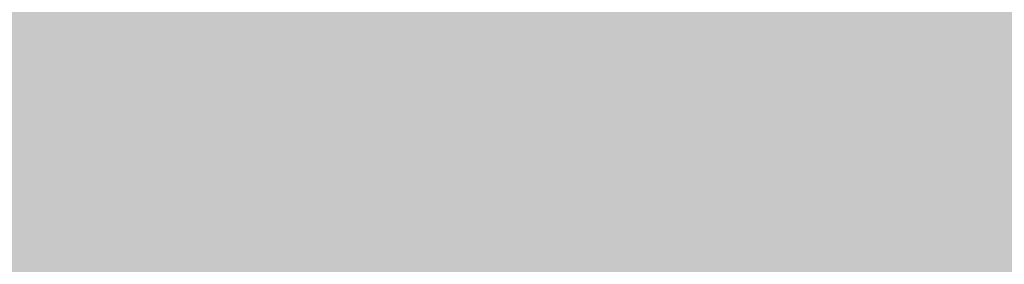
# Model space of a CAD drawing. Units: inches. Extents: x 2083 to 3317, y 1141 to 2115.
# Tile 158 of 256: x 3126.955939 to 3126.958245, y 1263.261932 to 1263.262504. Entities that reach past the tile are written whole.
import ezdxf

# ---------------------------------------------------------------- set-up
doc = ezdxf.new("R2010")
doc.units = ezdxf.units.IN
doc.layers.add('A-ANNO-DIMS', color=2, linetype='Continuous', lineweight=18)
doc.layers.add('A-WALL-PATT', color=251, linetype='Continuous', lineweight=13, true_color=0x636466)
doc.styles.get("Standard").update_dxf_attribs({"font": 'arial.ttf'})
doc.dimstyles.new('ISO-25', dxfattribs={"dimtxt": 12, "dimasz": 12, "dimexe": 1.25, "dimexo": 0.625, "dimtad": 1, "dimlunit": 3, "dimtxsty": 'Standard', "dimcen": 2.5, "dimadec": 0, "dimazin": 0, "dimtfac": 1, "dimtmove": 0, "dimatfit": 3, "dimfxl": 1, "dimarcsym": 0})

# ---------------------------------------------------------------- blocks, each defined once
blk = doc.blocks.new('*D26')
at = {"layer": 'A-ANNO-DIMS', "color": 0, "lineweight": -2, "transparency": 16777216}
for p, q in [((3088.985844, 1274.915092), (3088.985844, 1270.9519631)), ((3111.2400366, 1274.915092), (3111.2400366, 1270.9519631)), ((3076.985844, 1272.2019631), (2840.262447, 1272.2019631)), ((3111.2400366, 1272.2019631), (3088.985844, 1272.2019631)), ((3123.2400366, 1272.2019631), (3135.2400366, 1272.2019631))]:
    blk.add_line(p, q, dxfattribs=at)
at = {"layer": 'A-ANNO-DIMS', "color": 0, "transparency": 16777216}
for points in [[(3076.985844, 1274.2019631), (3076.985844, 1270.2019631), (3088.985844, 1272.2019631)], [(3123.2400366, 1274.2019631), (3123.2400366, 1270.2019631), (3111.2400366, 1272.2019631)]]:
    blk.add_solid(points, dxfattribs=at)
at = {"layer": 'Defpoints', "color": 0, "transparency": 16777216}
for p in [(3088.985844, 1275.540092), (3111.2400366, 1275.540092), (3088.985844, 1272.2019631)]:
    blk.add_point(p, dxfattribs=at)
at = {"layer": 'A-ANNO-DIMS', "color": 0, "transparency": 16777216, "insert": (2952.6241455, 1279.0316016), "char_height": 12, "attachment_point": 5}
blk.add_mtext('NIGHTSTAND 1\'-10 1/2" TYP.', dxfattribs=at)

msp = doc.modelspace()

# ---------------------------------------------------------------- hatches: boundary and pattern name
at = {"layer": 'A-WALL-PATT'}
h = msp.add_hatch(color=256, dxfattribs=at)
h.dxf.hatch_style = 1
h.paths.add_polyline_path([(3126.9597832, 2020.7613601), (2748.9597832, 2020.7613601), (2604.9597832, 2020.7613601), (2226.9597832, 2020.7613601), (2226.9597832, 1702.7613601), (2466.9597832, 1702.7613601), (2466.9597832, 1582.7613601), (2418.9597832, 1582.7613601), (2418.9597832, 1477.7613601), (2226.9597832, 1477.7613601), (2226.9597832, 1263.2613601), (2544.9597832, 1263.2613601), (2544.9597832, 1411.7613601), (2604.9597832, 1411.7613601), (2685.9597832, 1411.7613601), (2685.9597832, 1420.7613601), (2604.9597832, 1420.7613601), (2604.9597832, 1573.7613601), (2604.9597832, 1702.7613601), (2604.9597832, 2011.7613601), (2748.9597832, 2011.7613601), (2748.9597832, 1702.7613601), (2862.9597832, 1702.7613601), (2862.9597832, 1621.7613601), (2871.9597832, 1621.7613601), (2871.9597832, 1702.7613601), (2883.9597832, 1702.7613601), (2883.9597832, 1706.9394595, -0.026459), (2883.9597832, 1711.7613601), (2757.9597832, 1711.7613601), (2757.9597832, 1807.7613601), (2787.9597832, 1807.7613601), (2787.9597832, 1812.2613601), (2757.9597832, 1812.2613601), (2757.9597832, 2011.7613601), (2877.9597832, 2011.7613601), (2877.9597832, 1812.2613601), (2847.9597832, 1812.2613601), (2847.9597832, 1807.7613601), (2889.8357425, 1807.7613601), (2889.8357425, 1812.2613601), (2882.4597832, 1812.2613601), (2882.4597832, 2011.7613601), (3117.9597832, 2011.7613601), (3117.9597832, 1812.2613601), (2937.8357425, 1812.2613601), (2937.8357425, 1807.7613601), (2995.7097832, 1807.7613601), (2995.7097832, 1796.1176655), (3000.2097832, 1796.1176655), (3000.2097832, 1807.7613601), (3117.9597832, 1807.7613601), (3117.9597832, 1711.7613601), (3000.2097832, 1711.7613601), (3000.2097832, 1760.1176655), (2998.5727047, 1760.1176655, -0.020711), (2995.7097832, 1760.1176655), (2995.7097832, 1711.7613601), (2931.9597832, 1711.7613601), (2931.9597832, 1702.7613601), (3126.9597832, 1702.7613601)])
h.paths.add_polyline_path([(2471.4597832, 2011.7613601), (2471.4597832, 1810.0113601), (2462.7169357, 1810.0113601), (2462.7169357, 1805.5113601), (2505.9597832, 1805.5113601), (2505.9597832, 1810.0113601), (2475.9597832, 1810.0113601), (2475.9597832, 2011.7613601), (2595.9597832, 2011.7613601), (2595.9597832, 1810.0113601), (2565.9597832, 1810.0113601), (2565.9597832, 1805.5113601), (2595.9597832, 1805.5113601), (2595.9597832, 1711.7613601), (2235.9597832, 1711.7613601), (2235.9597832, 1805.5113601), (2353.7097832, 1805.5113601), (2353.7097832, 1796.0541624), (2358.2097832, 1796.0541624), (2358.2097832, 1805.5113601), (2414.7169357, 1805.5113601), (2414.7169357, 1810.0113601), (2235.9597832, 1810.0113601), (2235.9597832, 2011.7613601)], flags=16)
h.paths.add_polyline_path([(2270.2047343, 1994.6100082), (2270.2047343, 1970.6100082), (2246.2047343, 1970.6100082), (2246.2047343, 1994.6100082)], flags=0)
edge = h.paths.add_edge_path(flags=0)
edge.add_ellipse((2332.027391, 1899.7981761), major_axis=(-3.0429938, 3.0429938), ratio=0.16825245, start_angle=-161.3321656, end_angle=-156.3071136, ccw=False)
edge.add_ellipse((2333.0820373, 1898.7435297), major_axis=(-1.0546463, 1.0546463), ratio=0.453532097, start_angle=-123.371019, end_angle=-94.1591066)
edge = h.paths.add_edge_path(flags=0)
edge.add_ellipse((2332.027391, 1968.8762897), major_axis=(3.0429938, 3.0429938), ratio=0.16825245, start_angle=18.6678344, end_angle=23.6928864)
edge.add_spline(control_points=[(2332.9255964, 1970.6911045), (2332.2267681, 1970.3360997), (2330.8937087, 1969.6589054), (2328.4130803, 1970.9321376), (2327.2039345, 1967.7487119), (2324.7095965, 1969.9555886), (2322.5328223, 1967.012354), (2320.0128462, 1971.2958124), (2317.6803077, 1968.1578449), (2316.0405263, 1967.1020468), (2315.4269045, 1966.8096022)], knot_values=[0, 0, 0, 0, 2.267059, 4.324559, 6.685584, 8.878641, 11.121502, 14.300359, 17.755284, 19.732645, 19.732645, 19.732645, 19.732645], degree=3, periodic=0)
edge.add_ellipse((2332.027391, 1968.8762897), major_axis=(3.0429938, 3.0429938), ratio=0.16825245, start_angle=18.6678344, end_angle=23.6928864, ccw=False)
edge.add_ellipse((2333.0820373, 1969.930936), major_axis=(1.0546463, 1.0546463), ratio=0.453532097, start_angle=56.628981, end_angle=85.8408934, ccw=False)
edge = h.paths.add_edge_path(flags=0)
edge.add_spline(control_points=[(2296.4282874, 1967.9879081), (2293.6278045, 1965.3363137), (2287.7036238, 1959.727094), (2299.7438601, 1949.9956993), (2294.5325909, 1935.6685275), (2290.5732281, 1920.6035119), (2293.3941244, 1909.9736911), (2296.1854073, 1904.9665431)], knot_values=[0.099185, 0.099185, 0.099185, 0.099185, 0.345301, 0.619822, 0.982653, 1.386093, 1.810555, 1.810555, 1.810555, 1.810555], degree=3, periodic=0)
edge.add_spline(control_points=[(2296.1854073, 1904.9665431), (2297.3835817, 1902.6193002), (2298.0009694, 1901.9493116), (2298.5529698, 1901.4681549)], knot_values=[0.006246, 0.006246, 0.006246, 0.006246, 0.055476, 0.055476, 0.055476, 0.055476], degree=3, periodic=0)
edge.add_spline(control_points=[(2298.5529698, 1901.4681549), (2297.2586121, 1900.9232238), (2295.2252939, 1900.2321257), (2293.0602287, 1900.6142053), (2292.1014227, 1900.788415), (2292.0895776, 1900.790568)], knot_values=[0.312835, 0.312835, 0.312835, 0.312835, 0.40178, 0.474987, 0.475903, 0.475903, 0.475903, 0.475903], degree=3, periodic=0)
edge.add_arc((2292.7936464, 1904.6641088), 3.9370079, 215.4208969, 259.6981795, ccw=False)
edge.add_spline(control_points=[(2289.5853139, 1902.3823039), (2289.4766524, 1902.5350874), (2289.3684805, 1902.6880353), (2289.2608648, 1902.8411699)], knot_values=[0.102872, 0.102872, 0.102872, 0.102872, 0.116896, 0.116896, 0.116896, 0.116896], degree=3, periodic=0)
edge.add_spline(control_points=[(2289.2608648, 1902.8411699), (2288.6866042, 1902.5501922), (2287.6400477, 1902.0199025), (2285.8813368, 1901.8739536), (2283.8529717, 1901.5043521), (2281.7199871, 1899.7105375), (2278.4669913, 1899.492942), (2276.1571361, 1901.8832022), (2272.2589526, 1899.8040711), (2267.7776054, 1901.8431828), (2262.2438819, 1900.1840326), (2257.414927, 1901.7820606), (2254.318374, 1900.7261196), (2253.1782849, 1900.3373431)], knot_values=[0, 0, 0, 0, 1.907977, 3.477176, 5.261074, 7.972851, 11.680248, 13.717921, 16.939592, 22.789562, 27.502503, 33.595215, 37.145618, 37.145618, 37.145618, 37.145618], degree=3, periodic=0)
edge.add_line((2253.1782849, 1900.3373431), (2250.2442397, 1902.8411699))
edge.add_line((2250.2442397, 1902.8411699), (2250.2442397, 1965.8332959))
edge.add_line((2250.2442397, 1965.8332959), (2253.1782849, 1968.3371226))
edge.add_spline(control_points=[(2253.1782849, 1968.3371226), (2254.318374, 1967.9483462), (2257.414927, 1966.8924051), (2262.2438819, 1968.4904332), (2267.7776054, 1966.8312829), (2271.5267301, 1968.5372172), (2273.8759143, 1967.8282895), (2274.2067012, 1967.7276424)], knot_values=[0, 0, 0, 0, 0.09018, 0.244935, 0.364644, 0.513233, 0.537855, 0.537855, 0.537855, 0.537855], degree=3, periodic=0)
edge.add_arc((2274.3528869, 1963.7933495), 3.9370079, 72.0511336, 92.1279492, ccw=False)
edge.add_arc((2281.2969331, 1985.2300027), 18.5962982, 252.05113361, 288.56572166)
edge.add_arc((2292.3167172, 1956.0288805), 12.6460805, 71.02678788, 113.77821843, ccw=False)
edge = h.paths.add_edge_path(flags=0)
edge.add_spline(control_points=[(2274.8994147, 1951.8561946), (2275.066156, 1951.6165924), (2275.2326866, 1951.3765878), (2275.3979871, 1951.1358545)], knot_values=[1.409916, 1.409916, 1.409916, 1.409916, 1.43159, 1.43159, 1.43159, 1.43159], degree=3, periodic=0)
edge.add_spline(control_points=[(2275.3979871, 1951.1358545), (2275.7921055, 1950.5618854), (2276.1792311, 1949.9837745), (2276.5455462, 1949.3971029)], knot_values=[1.358238, 1.358238, 1.358238, 1.358238, 1.409916, 1.409916, 1.409916, 1.409916], degree=3, periodic=0)
edge.add_line((2276.5455462, 1949.3971029), (2277.437289, 1947.8621847))
edge.add_spline(control_points=[(2277.437289, 1947.8621847), (2276.3038341, 1945.6731147), (2274.6396979, 1942.4268817), (2274.631615, 1938.0938998), (2272.7991237, 1930.8515498), (2274.3564261, 1943.8970461), (2275.9476814, 1947.9233558), (2276.5455462, 1949.3971029)], knot_values=[0.005632, 0.005632, 0.005632, 0.005632, 0.186014, 0.266002, 0.357087, 0.59639, 0.739732, 0.739732, 0.739732, 0.739732], degree=3, periodic=0)
edge.add_spline(control_points=[(2276.5455462, 1949.3971029), (2276.1792311, 1949.9837745), (2275.7921055, 1950.5618854), (2275.3979871, 1951.1358545)], knot_values=[1.358238, 1.358238, 1.358238, 1.358238, 1.409916, 1.409916, 1.409916, 1.409916], degree=3, periodic=0)
edge.add_spline(control_points=[(2275.3979871, 1951.1358545), (2274.9425002, 1950.0804523), (2274.2077604, 1948.0252718), (2273.9346018, 1944.8514774), (2272.4685341, 1937.6274891), (2273.4662155, 1945.6964663), (2274.7006154, 1951.0594725), (2274.8994147, 1951.8561946)], knot_values=[0.104364, 0.104364, 0.104364, 0.104364, 0.189636, 0.269624, 0.36071, 0.600013, 0.644622, 0.644622, 0.644622, 0.644622], degree=3, periodic=0)
h.paths.add_polyline_path([(2269.1675139, 1963.1275729, -0.357527), (2268.170633, 1960.9763695, -0.092561), (2268.170633, 1939.4363249, -0.357527), (2269.1675139, 1937.2851215, -0.357527), (2267.0163105, 1938.2820024, -0.164785), (2254.6855813, 1938.2820024, -0.357527), (2252.5343779, 1937.2851215, -0.357527), (2253.5312587, 1939.4363249, -0.092561), (2253.5312587, 1960.9763695, -0.357527), (2252.5343779, 1963.1275729, -0.357527), (2254.6855813, 1962.130692, -0.164785), (2267.0163105, 1962.130692, -0.357527)], flags=0)
h.paths.add_polyline_path([(2248.8740679, 1967.8017998), (2248.8740679, 1957.0277095), (2249.4577833, 1957.0277095), (2249.4577833, 1911.6467562), (2248.8740679, 1911.6467562), (2248.8740679, 1900.8726659), (2246.5118632, 1900.8726659, 0.197327), (2244.1496584, 1902.4568734), (2244.1496584, 1966.2175923, 0.197327), (2246.5118632, 1967.8017998)], flags=0)
h.paths.add_polyline_path([(2269.1675139, 1931.3893442, -0.357527), (2268.170633, 1929.2381408, -0.092561), (2268.170633, 1907.6980962, -0.357527), (2269.1675139, 1905.5468928, -0.357527), (2267.0163105, 1906.5437737, -0.164785), (2254.6855813, 1906.5437737, -0.357527), (2252.5343779, 1905.5468928, -0.357527), (2253.5312587, 1907.6980962, -0.092561), (2253.5312587, 1929.2381408, -0.357527), (2252.5343779, 1931.3893442, -0.357527), (2254.6855813, 1930.3924634, -0.164785), (2267.0163105, 1930.3924634, -0.357527)], flags=0)
edge = h.paths.add_edge_path(flags=0)
edge.add_spline(control_points=[(2276.1968578, 1906.7237016), (2276.1681442, 1909.0289278), (2276.1140492, 1913.371852), (2270.5984171, 1924.9249783), (2273.9051746, 1919.0127787), (2275.9217115, 1916.2620626), (2275.4745699, 1912.4021495), (2277.2578735, 1910.3806206), (2276.6960436, 1908.2250358), (2276.6462176, 1906.8130226), (2276.6178249, 1906.0084068)], knot_values=[0, 0, 0, 0, 8.61026, 16.221274, 18.843057, 23.804898, 27.440828, 29.356102, 31.203478, 33.650687, 33.650687, 33.650687, 33.650687], degree=3, periodic=0)
edge.add_spline(control_points=[(2276.6178249, 1906.0084068), (2276.6233131, 1905.6241436), (2276.4977381, 1904.6286608), (2275.4417789, 1903.8547251), (2274.9373144, 1903.0804497), (2274.8590804, 1902.8411699)], knot_values=[0.156488, 0.156488, 0.156488, 0.156488, 0.184398, 0.231376, 0.250598, 0.250598, 0.250598, 0.250598], degree=3, periodic=0)
edge.add_line((2274.8590804, 1902.8411699), (2276.50598, 1902.8411699))
edge.add_spline(control_points=[(2276.50598, 1902.8411699), (2276.7883084, 1903.0849395), (2277.6650711, 1904.1251958), (2278.2495378, 1904.340738), (2277.6538719, 1908.5273866), (2278.15567, 1906.2278078), (2278.100464, 1905.2859484), (2278.8466748, 1904.0690054), (2277.8567853, 1903.4149482), (2277.8741909, 1902.9910497), (2277.9035616, 1902.8411699)], knot_values=[0.059574, 0.059574, 0.059574, 0.059574, 0.080753, 0.103741, 0.16972, 0.176036, 0.207137, 0.240474, 0.262341, 0.27366, 0.27366, 0.27366, 0.27366], degree=3, periodic=0)
edge.add_line((2277.9035616, 1902.8411699), (2280.0298255, 1902.8411699))
edge.add_spline(control_points=[(2280.0298255, 1902.8411699), (2279.8882214, 1903.088398), (2279.4992571, 1903.9815512), (2280.1522839, 1905.9393491), (2278.103615, 1909.6577572), (2279.7623946, 1907.185285), (2280.3279002, 1904.8748608), (2280.4851086, 1903.4895904), (2281.4632687, 1903.2494323), (2281.7583431, 1902.9364967), (2281.8340361, 1902.8411699)], knot_values=[0.013856, 0.013856, 0.013856, 0.013856, 0.034874, 0.088867, 0.107879, 0.126738, 0.158714, 0.193757, 0.217487, 0.226722, 0.226722, 0.226722, 0.226722], degree=3, periodic=0)
edge.add_spline(control_points=[(2281.8340361, 1902.8411699), (2281.7875348, 1902.8267029), (2281.6470224, 1902.7829881), (2281.3955272, 1902.85949), (2281.088077, 1902.9852418), (2280.7206826, 1903.060902), (2280.3334513, 1903.0257257), (2280.1247668, 1902.898879), (2280.0298255, 1902.8411699)], knot_values=[0, 0, 0, 0, 0.14413, 0.435517, 0.749276, 1.153046, 1.548371, 1.878348, 1.878348, 1.878348, 1.878348], degree=3, periodic=0)
edge.add_line((2280.0298255, 1902.8411699), (2277.9035616, 1902.8411699))
edge.add_spline(control_points=[(2277.9035616, 1902.8411699), (2277.892855, 1902.7958553), (2277.865396, 1902.6796374), (2277.6074793, 1902.6874828), (2277.2740503, 1902.8006999), (2276.8379209, 1902.6197745), (2276.5838074, 1902.7892611), (2276.50598, 1902.8411699)], knot_values=[0, 0, 0, 0, 0.127189, 0.326199, 0.628009, 1.24357, 1.515331, 1.515331, 1.515331, 1.515331], degree=3, periodic=0)
edge.add_line((2276.50598, 1902.8411699), (2274.8590804, 1902.8411699))
edge.add_spline(control_points=[(2274.8590804, 1902.8411699), (2274.8144367, 1902.8985868), (2274.7251297, 1903.013446), (2274.4934765, 1903.1189684), (2274.2442854, 1902.9605386), (2273.9371207, 1903.1849416), (2273.6140395, 1902.9831428), (2273.4083164, 1902.8830449), (2273.322254, 1902.8411699)], knot_values=[0, 0, 0, 0, 0.21843, 0.436957, 0.687977, 0.990379, 1.398396, 1.69185, 1.69185, 1.69185, 1.69185], degree=3, periodic=0)
edge.add_spline(control_points=[(2273.322254, 1902.8411699), (2273.6167403, 1903.445692), (2274.2739977, 1904.5382529), (2276.0272387, 1904.5737017), (2276.2069634, 1906.5836372), (2276.1968578, 1906.7237016)], knot_values=[0.012227, 0.012227, 0.012227, 0.012227, 0.059472, 0.106218, 0.134458, 0.134458, 0.134458, 0.134458], degree=3, periodic=0)
h.paths.add_polyline_path([(2270.7760538, 1897.7898284), (2270.7760538, 1873.7898284), (2246.7760538, 1873.7898284), (2246.7760538, 1897.7898284)], flags=0)
h.paths.add_polyline_path([(2353.7097832, 1760.0050593), (2353.7097832, 1760.0541624), (2358.2097832, 1760.0541624, -0.033729)], flags=0)
h.paths.add_polyline_path([(2321.8191188, 1737.5291862), (2341.9953271, 1737.5291862, -0.414214), (2343.2032727, 1736.3212406), (2343.2032727, 1721.0205964, -0.414214), (2341.9953271, 1719.8126508), (2321.8191188, 1719.8126508, -0.414214), (2320.6111732, 1721.0205964), (2320.6111732, 1736.3212406, -0.414214)], flags=0)
h.paths.add_polyline_path([(2324.2350099, 1736.3212406), (2339.5794359, 1736.3212406, -0.414214), (2341.9953271, 1733.9053494), (2341.9953271, 1725.4497302, -0.414214), (2339.5794359, 1723.033839), (2333.6805885, 1723.033839), (2333.8453172, 1722.0454666, -0.870646), (2335.4253988, 1721.8258934, -0.767327), (2333.922694, 1721.4232449), (2331.2910241, 1721.4232449, -0.767327), (2329.7883193, 1721.8258934, -0.870646), (2331.3684009, 1722.0454666), (2331.5331296, 1723.033839), (2324.2350099, 1723.033839, -0.414214), (2321.8191188, 1725.4497302), (2321.8191188, 1733.9053494, -0.414214)], flags=0)
h.paths.add_polyline_path([(2570.4837892, 1928.6154443), (2589.6837892, 1928.6154443), (2590.1688286, 1928.6154443), (2590.1688286, 1904.9933971), (2570.4837892, 1904.9933971)], flags=0)
h.paths.add_polyline_path([(2574.4473242, 1927.2638215, -1), (2572.8288357, 1927.2638215, -1)], flags=0)
h.paths.add_polyline_path([(2573.0898665, 1926.9408768), (2573.925032, 1927.7760423), (2574.1477428, 1927.5533315), (2573.3125773, 1926.718166)], flags=0)
h.paths.add_polyline_path([(2578.7790648, 1919.7296175, -1), (2571.5916632, 1919.7296175, -1)], flags=0)
h.paths.add_polyline_path([(2578.385364, 1919.7296175, -1), (2571.985364, 1919.7296175, -1)], flags=0)
h.paths.add_polyline_path([(2331.5957638, 1729.4762156, -1), (2333.6179542, 1729.4762156, -1)], flags=0)
h.paths.add_polyline_path([(2578.0342282, 1927.2638215, -1), (2576.4157396, 1927.2638215, -1)], flags=0)
h.paths.add_polyline_path([(2576.6888513, 1927.5310886), (2576.9115621, 1927.7537993), (2577.7467276, 1926.9186339), (2577.5240168, 1926.6959231)], flags=0)
h.paths.add_polyline_path([(2578.1390648, 1909.8595388, -1), (2572.2316632, 1909.8595388, -1)], flags=0)
h.paths.add_polyline_path([(2577.745364, 1909.8595388, -1), (2572.625364, 1909.8595388, -1)], flags=0)
h.paths.add_polyline_path([(2583.7977179, 1927.2638215, -1), (2582.1792294, 1927.2638215, -1)], flags=0)
h.paths.add_polyline_path([(2582.7186487, 1927.7537993), (2583.5538142, 1926.9186339), (2583.3311034, 1926.6959231), (2582.4959379, 1927.5310886)], flags=0)
h.paths.add_polyline_path([(2582.4959379, 1927.5310886), (2582.7186487, 1927.7537993), (2583.5538142, 1926.9186339), (2583.3311034, 1926.6959231)], flags=0)
h.paths.add_polyline_path([(2587.7390648, 1920.5296175, -1), (2581.8316632, 1920.5296175, -1)], flags=0)
h.paths.add_polyline_path([(2587.345364, 1920.5296175, -1), (2582.225364, 1920.5296175, -1)], flags=0)
h.paths.add_polyline_path([(2587.3846219, 1927.2638215, -1), (2585.7661333, 1927.2638215, -1)], flags=0)
h.paths.add_polyline_path([(2586.0819925, 1926.9802469), (2586.917158, 1927.8154124), (2587.1398688, 1927.5927016), (2586.3047033, 1926.7575361)], flags=0)
h.paths.add_polyline_path([(2588.3790648, 1910.6595388, -1), (2581.1916632, 1910.6595388, -1)], flags=0)
h.paths.add_polyline_path([(2587.985364, 1910.6595388, -1), (2581.585364, 1910.6595388, -1)], flags=0)
h.paths.add_polyline_path([(2417.1677288, 1729.4778955), (2437.3439372, 1729.4778955, -0.414214), (2438.5518828, 1728.2699499), (2438.5518828, 1712.9693057, -0.414214), (2437.3439372, 1711.7613601), (2417.1677288, 1711.7613601, -0.414214), (2415.9597832, 1712.9693057), (2415.9597832, 1728.2699499, -0.414214)], flags=0)
h.paths.add_polyline_path([(2419.58362, 1728.2699499), (2434.928046, 1728.2699499, -0.414214), (2437.3439372, 1725.8540587), (2437.3439372, 1717.3984395, -0.414214), (2434.928046, 1714.9825483), (2429.0291985, 1714.9825483), (2429.1939273, 1713.9941758, -0.870646), (2430.7740089, 1713.7746027, -0.767327), (2429.2713041, 1713.3719542), (2426.6396342, 1713.3719542, -0.767327), (2425.1369294, 1713.7746027, -0.870646), (2426.717011, 1713.9941758), (2426.8817397, 1714.9825483), (2419.58362, 1714.9825483, -0.414214), (2417.1677288, 1717.3984395), (2417.1677288, 1725.8540587, -0.414214)], flags=0)
h.paths.add_polyline_path([(2419.58362, 1728.2699499), (2434.928046, 1728.2699499, -0.414214), (2437.3439372, 1725.8540587), (2437.3439372, 1717.3984395, -0.414214), (2434.928046, 1714.9825483), (2429.0291985, 1714.9825483), (2428.3581177, 1719.0090337), (2427.5528206, 1719.0090337), (2426.8817397, 1714.9825483), (2419.58362, 1714.9825483, -0.414214), (2417.1677288, 1717.3984395), (2417.1677288, 1725.8540587, -0.414214)], flags=0)
h.paths.add_polyline_path([(2426.9443739, 1721.4249248, -1), (2428.9665643, 1721.4249248, -1)], flags=0)
h.paths.add_polyline_path([(2475.9597832, 1702.7613601), (2595.9597832, 1702.7613601), (2595.9597832, 1582.7613601), (2475.9597832, 1582.7613601)], flags=16)
h.paths.add_polyline_path([(2427.9597832, 1573.7613601), (2595.9597832, 1573.7613601), (2595.9597832, 1468.7613601), (2595.9597832, 1420.7613601), (2384.4597832, 1420.7613601), (2384.4597832, 1468.7613601), (2427.9597832, 1468.7613601)], flags=16)
h.paths.add_polyline_path([(2379.9597832, 1468.7613601), (2379.9597832, 1420.7613601), (2235.9597832, 1420.7613601), (2235.9597832, 1468.7613601)], flags=16)
h.paths.add_polyline_path([(2317.8159962, 1466.695767), (2337.9922045, 1466.695767, -0.414214), (2339.2001501, 1465.4878214), (2339.2001501, 1450.1871771, -0.414214), (2337.9922045, 1448.9792315), (2317.8159962, 1448.9792315, -0.414214), (2316.6080506, 1450.1871771), (2316.6080506, 1465.4878214, -0.414214)], flags=0)
h.paths.add_polyline_path([(2320.2318874, 1465.4878214), (2335.5763133, 1465.4878214, -0.414214), (2337.9922045, 1463.0719302), (2337.9922045, 1454.616311, -0.414214), (2335.5763133, 1452.2004198), (2329.6774659, 1452.2004198), (2329.8421946, 1451.2120473, -0.870646), (2331.4222762, 1450.9924742, -0.767327), (2329.9195714, 1450.5898257), (2327.2879015, 1450.5898257, -0.767327), (2325.7851967, 1450.9924742, -0.870646), (2327.3652783, 1451.2120473), (2327.530007, 1452.2004198), (2320.2318874, 1452.2004198, -0.414214), (2317.8159962, 1454.616311), (2317.8159962, 1463.0719302, -0.414214)], flags=0)
h.paths.add_polyline_path([(2320.2318874, 1465.4878214), (2335.5763133, 1465.4878214, -0.414214), (2337.9922045, 1463.0719302), (2337.9922045, 1454.616311, -0.414214), (2335.5763133, 1452.2004198), (2329.6774659, 1452.2004198), (2329.006385, 1456.2269051), (2328.2010879, 1456.2269051), (2327.530007, 1452.2004198), (2320.2318874, 1452.2004198, -0.414214), (2317.8159962, 1454.616311), (2317.8159962, 1463.0719302, -0.414214)], flags=0)
h.paths.add_polyline_path([(2327.5926413, 1458.6427963, -1), (2329.6148317, 1458.6427963, -1)], flags=0)
h.paths.add_polyline_path([(2244.4117436, 1433.3404531), (2241.9209449, 1433.3404531, -0.414214), (2240.0178562, 1435.2435418), (2240.0178562, 1440.9528078, -0.414211), (2241.920925, 1442.8558965), (2244.4117436, 1442.8558965, -1.976472)], flags=0)
h.paths.add_polyline_path([(2245.3568884, 1434.3975358, -0.414214), (2245.3568884, 1441.7988138, -2.144098)], flags=0)
h.paths.add_polyline_path([(2535.9597832, 1416.2613601), (2535.9597832, 1272.2613601), (2235.9597832, 1272.2613601), (2235.9597832, 1416.2613601)], flags=16)
h.paths.add_polyline_path([(2260.1195614, 1384.2928413), (2260.1195614, 1362.0386487), (2237.8653688, 1362.0386487), (2237.8653688, 1384.2928413)], flags=0)
edge = h.paths.add_edge_path(flags=0)
edge.add_line((2318.2518466, 1362.0932983), (2318.1457968, 1362.0009726))
edge.add_ellipse((2317.4451158, 1360.4310442), major_axis=(2.8216404, 2.8216404), ratio=0.16825245, start_angle=18.6678344, end_angle=20.9481273, ccw=False)
edge.add_ellipse((2318.4230451, 1361.4089735), major_axis=(0.9779293, 0.9779293), ratio=0.453532097, start_angle=56.628981, end_angle=70.2262012, ccw=False)
edge = h.paths.add_edge_path(flags=0)
edge.add_line((2319.1073699, 1295.5710784), (2319.0150442, 1295.6771282))
edge.add_ellipse((2317.4451158, 1296.3778091), major_axis=(-2.8216404, 2.8216404), ratio=0.16825245, start_angle=-161.3321656, end_angle=-159.0518727, ccw=False)
edge.add_ellipse((2318.4230451, 1295.3998798), major_axis=(-0.9779293, 0.9779293), ratio=0.453532097, start_angle=-123.371019, end_angle=-109.7737988)
edge = h.paths.add_edge_path(flags=0)
edge.add_spline(control_points=[(2284.2103489, 1301.1702189), (2284.5806878, 1300.444719), (2284.8911891, 1299.8920243), (2285.159553, 1299.4610182)], knot_values=[0.039066, 0.039066, 0.039066, 0.039066, 0.055476, 0.055476, 0.055476, 0.055476], degree=3, periodic=0)
edge.add_line((2285.159553, 1299.4610182), (2284.2103489, 1301.1702189))
edge = h.paths.add_edge_path(flags=0)
edge.add_line((2280.4124579, 1297.2980125), (2283.3699905, 1297.0361216))
edge.add_line((2283.3699905, 1297.0361216), (2286.4056902, 1297.9263104))
edge.add_spline(control_points=[(2286.4056902, 1297.9263104), (2285.305487, 1297.4631193), (2284.3447774, 1297.1291508), (2283.3699905, 1297.0361216)], knot_values=[0.394369, 0.394369, 0.394369, 0.394369, 0.475903, 0.475903, 0.475903, 0.475903], degree=3, periodic=0)
edge.add_spline(control_points=[(2283.3699905, 1297.0361216), (2283.2813895, 1297.027666), (2282.316289, 1296.9573356), (2281.3125019, 1297.1344787), (2280.4234414, 1297.2960161), (2280.4124579, 1297.2980125)], knot_values=[0.312835, 0.312835, 0.312835, 0.312835, 0.320246, 0.393453, 0.394369, 0.394369, 0.394369, 0.394369], degree=3, periodic=0)
edge = h.paths.add_edge_path(flags=0)
edge.add_line((2284.4355615, 1359.6072854), (2280.4462909, 1355.328047))
edge.add_line((2280.4462909, 1355.328047), (2279.5799868, 1351.0177544))
edge.add_line((2279.5799868, 1351.0177544), (2282.4129737, 1346.5804327))
edge.add_spline(control_points=[(2282.4129737, 1346.5804327), (2283.1533308, 1345.5892358), (2284.2528957, 1344.0288973), (2284.801037, 1342.3871671), (2284.9351625, 1341.8055443)], knot_values=[1.240098, 1.240098, 1.240098, 1.240098, 1.332892, 1.382712, 1.382712, 1.382712, 1.382712], degree=3, periodic=0)
edge.add_spline(control_points=[(2284.9351625, 1341.8055443), (2285.3191079, 1340.1406002), (2285.2330291, 1338.4092041), (2284.9099384, 1336.6541222)], knot_values=[1.097484, 1.097484, 1.097484, 1.097484, 1.240098, 1.240098, 1.240098, 1.240098], degree=3, periodic=0)
edge.add_spline(control_points=[(2284.9099384, 1336.6541222), (2284.5868478, 1334.8990403), (2284.0267453, 1333.1202725), (2283.4626437, 1331.3605849)], knot_values=[0.95487, 0.95487, 0.95487, 0.95487, 1.097484, 1.097484, 1.097484, 1.097484], degree=3, periodic=0)
edge.add_line((2283.4626437, 1331.3605849), (2281.8903759, 1326.153357))
edge.add_line((2281.8903759, 1326.153357), (2280.7562592, 1321.0560888))
edge.add_line((2280.7562592, 1321.0560888), (2280.2992048, 1316.0019772))
edge.add_line((2280.2992048, 1316.0019772), (2280.7159327, 1310.9500678))
edge.add_line((2280.7159327, 1310.9500678), (2282.0280939, 1305.9721367))
edge.add_line((2282.0280939, 1305.9721367), (2284.2103489, 1301.1702189))
edge.add_spline(control_points=[(2284.2103489, 1301.1702189), (2283.3407305, 1302.7301854), (2282.6119044, 1304.3364933), (2282.0280939, 1305.9721367)], knot_values=[0.099185, 0.099185, 0.099185, 0.099185, 0.241799, 0.241799, 0.241799, 0.241799], degree=3, periodic=0)
edge.add_spline(control_points=[(2282.0280939, 1305.9721367), (2281.4442835, 1307.6077801), (2281.0054886, 1309.2727591), (2280.7159327, 1310.9500678)], knot_values=[0.241799, 0.241799, 0.241799, 0.241799, 0.384413, 0.384413, 0.384413, 0.384413], degree=3, periodic=0)
edge.add_spline(control_points=[(2280.7159327, 1310.9500678), (2280.4332411, 1312.5876134), (2280.2893863, 1314.2769594), (2280.2988938, 1315.9620324), (2280.2992048, 1316.0019772)], knot_values=[0.384413, 0.384413, 0.384413, 0.384413, 0.523647, 0.527028, 0.527028, 0.527028, 0.527028], degree=3, periodic=0)
edge.add_spline(control_points=[(2280.2992048, 1316.0019772), (2280.3123257, 1317.6869552), (2280.4778706, 1319.3679256), (2280.7562592, 1321.0560888)], knot_values=[0.527028, 0.527028, 0.527028, 0.527028, 0.669642, 0.669642, 0.669642, 0.669642], degree=3, periodic=0)
edge.add_spline(control_points=[(2280.7562592, 1321.0560888), (2281.0346478, 1322.7442519), (2281.4258801, 1324.4396079), (2281.8903759, 1326.153357)], knot_values=[0.669642, 0.669642, 0.669642, 0.669642, 0.812256, 0.812256, 0.812256, 0.812256], degree=3, periodic=0)
edge.add_spline(control_points=[(2281.8903759, 1326.153357), (2282.2643834, 1327.5332507), (2282.7878702, 1329.2618097), (2283.352751, 1331.0177803), (2283.4626437, 1331.3605849)], knot_values=[0.812256, 0.812256, 0.812256, 0.812256, 0.927087, 0.95487, 0.95487, 0.95487, 0.95487], degree=3, periodic=0)
edge.add_line((2283.4626437, 1331.3605849), (2284.9099384, 1336.6541222))
edge.add_line((2284.9099384, 1336.6541222), (2284.9351625, 1341.8055443))
edge.add_line((2284.9351625, 1341.8055443), (2282.4129737, 1346.5804327))
edge.add_spline(control_points=[(2282.4129737, 1346.5804327), (2281.2751273, 1348.1037918), (2280.0784467, 1349.5703178), (2279.5799868, 1351.0177544)], knot_values=[1.382712, 1.382712, 1.382712, 1.382712, 1.525326, 1.525326, 1.525326, 1.525326], degree=3, periodic=0)
edge.add_spline(control_points=[(2279.5799868, 1351.0177544), (2279.4432818, 1351.4147209), (2279.1363124, 1352.856922), (2279.7351897, 1354.2903851), (2280.4462909, 1355.328047)], knot_values=[1.525326, 1.525326, 1.525326, 1.525326, 1.564439, 1.667941, 1.667941, 1.667941, 1.667941], degree=3, periodic=0)
edge.add_spline(control_points=[(2280.4462909, 1355.328047), (2281.4261132, 1356.7578354), (2282.9308373, 1358.1825604), (2284.4355615, 1359.6072854)], knot_values=[1.667941, 1.667941, 1.667941, 1.667941, 1.810555, 1.810555, 1.810555, 1.810555], degree=3, periodic=0)
edge.add_arc((2280.6230749, 1348.518181), 11.7261796, 71.02678788, 113.77821843)
edge.add_arc((2270.4048917, 1375.5951559), 17.2435667, 252.05113361, 288.56572166, ccw=False)
edge.add_arc((2263.9659692, 1355.7178471), 3.6506221, 72.0511336, 92.1279492)
edge.add_arc((2263.9659692, 1355.7178471), 3.6506221, 92.1279492, 177.98513)
edge.add_spline(control_points=[(2260.3176041, 1355.8461989), (2260.2604169, 1354.2206683), (2260.551278, 1350.1865469), (2262.9993445, 1346.7662507), (2264.4727415, 1344.6490245)], knot_values=[1.43159, 1.43159, 1.43159, 1.43159, 1.564144, 1.770695, 1.770695, 1.770695, 1.770695], degree=3, periodic=0)
edge.add_line((2264.4727415, 1344.6490245), (2264.9355904, 1343.9825301))
edge.add_spline(control_points=[(2263.8010444, 1340.2481052), (2263.8432379, 1340.5140884), (2264.0672444, 1341.7564652), (2264.5126928, 1343.0024532), (2264.9350468, 1343.9810834)], knot_values=[0.53657, 0.53657, 0.53657, 0.53657, 0.559349, 0.644622, 0.644622, 0.644622, 0.644622], degree=3, periodic=0)
edge.add_spline(control_points=[(2264.9350468, 1343.9810834), (2265.1177715, 1343.7149747), (2265.2988751, 1343.4479058), (2265.4767562, 1343.1793646)], knot_values=[1.384077, 1.384077, 1.384077, 1.384077, 1.409916, 1.409916, 1.409916, 1.409916], degree=3, periodic=0)
edge.add_spline(control_points=[(2265.4767562, 1343.1793646), (2265.6546373, 1342.9108234), (2265.8292958, 1342.64081), (2265.9991301, 1342.368812)], knot_values=[1.358238, 1.358238, 1.358238, 1.358238, 1.384077, 1.384077, 1.384077, 1.384077], degree=3, periodic=0)
edge.add_line((2265.9991301, 1342.368812), (2266.8260057, 1340.9455468))
edge.add_spline(control_points=[(2266.8260057, 1340.9455468), (2268.894401, 1337.0896912), (2271.3981727, 1325.8430009), (2270.5161644, 1310.5685568), (2275.9193759, 1301.860609), (2277.7895113, 1299.1994495)], knot_values=[0.116896, 0.116896, 0.116896, 0.116896, 0.472987, 1.050969, 1.313793, 1.313793, 1.313793, 1.313793], degree=3, periodic=0)
edge.add_spline(control_points=[(2277.7895113, 1299.1994495), (2277.8394051, 1299.1284519), (2277.8894277, 1299.0574975), (2277.9395717, 1298.9865839)], knot_values=[0.109884, 0.109884, 0.109884, 0.109884, 0.116896, 0.116896, 0.116896, 0.116896], degree=3, periodic=0)
edge.add_line((2277.9395717, 1298.9865839), (2277.7888489, 1299.1991139))
edge.add_spline(control_points=[(2277.7888489, 1299.1991139), (2277.2565819, 1298.9294144), (2276.2863504, 1298.4379024), (2275.0393517, 1298.3344186), (2274.3833299, 1298.2388951), (2274.2152543, 1298.209338)], knot_values=[33.12187, 33.12187, 33.12187, 33.12187, 35.029056, 36.598255, 37.144827, 37.144827, 37.144827, 37.144827], degree=3, periodic=0)
edge.add_line((2274.2152543, 1298.209338), (2273.073147, 1297.8929607))
edge.add_spline(control_points=[(2273.073147, 1297.8929607), (2272.3229363, 1297.579784), (2271.0391507, 1296.5105078), (2269.2483948, 1296.2260622), (2268.4231004, 1296.3746543)], knot_values=[26.532584, 26.532584, 26.532584, 26.532584, 29.198919, 31.839101, 31.839101, 31.839101, 31.839101], degree=3, periodic=0)
edge.add_line((2268.4231004, 1296.3746543), (2263.8785014, 1297.4575338))
edge.add_spline(control_points=[(2263.8785014, 1297.4575338), (2263.5560769, 1297.3594345), (2261.8603064, 1296.8386943), (2260.2387805, 1297.2824073), (2258.9334543, 1297.5164611)], knot_values=[15.919551, 15.919551, 15.919551, 15.919551, 16.939592, 21.226067, 21.226067, 21.226067, 21.226067], degree=3, periodic=0)
edge.add_line((2258.9334543, 1297.5164611), (2254.0552332, 1297.3290098))
edge.add_spline(control_points=[(2254.0552332, 1297.3290098), (2253.7555255, 1297.295815), (2252.1136834, 1297.1651738), (2250.4618687, 1297.5442209), (2249.1296862, 1297.6678818)], knot_values=[5.306517, 5.306517, 5.306517, 5.306517, 6.276435, 10.613034, 10.613034, 10.613034, 10.613034], degree=3, periodic=0)
edge.add_line((2249.1296862, 1297.6678818), (2244.3316495, 1296.8777561))
edge.add_line((2244.3316495, 1296.8777561), (2241.6110326, 1299.1994495))
edge.add_line((2241.6110326, 1299.1994495), (2241.6110326, 1357.6094038))
edge.add_line((2241.6110326, 1357.6094038), (2244.3316495, 1359.9310973))
edge.add_line((2244.3316495, 1359.9310973), (2252.7288228, 1359.5426917))
edge.add_spline(control_points=[(2252.7288228, 1359.5426917), (2252.8709387, 1359.5464396), (2253.3057402, 1359.5481716), (2253.7398447, 1359.5142744), (2254.0317419, 1359.4824261)], knot_values=[0.233291, 0.233291, 0.233291, 0.233291, 0.244935, 0.268927, 0.268927, 0.268927, 0.268927], degree=3, periodic=0)
edge.add_line((2254.0317419, 1359.4824261), (2259.5871899, 1359.4163899))
edge.add_spline(control_points=[(2259.5871899, 1359.4163899), (2260.6770676, 1359.6285026), (2262.0731971, 1359.8970025), (2263.5236925, 1359.4592776), (2263.8304173, 1359.3659518)], knot_values=[0.422516, 0.422516, 0.422516, 0.422516, 0.513233, 0.537855, 0.537855, 0.537855, 0.537855], degree=3, periodic=0)
edge.add_arc((2263.9659692, 1355.7178471), 3.6506221, 72.0511336, 92.1279492, ccw=False)
edge.add_arc((2270.4048917, 1375.5951559), 17.2435667, 252.05113361, 288.56572166)
edge.add_arc((2280.6230749, 1348.518181), 11.7261796, 71.02678788, 113.77821843, ccw=False)
h.paths.add_polyline_path([(2240.3405298, 1359.4347149), (2240.3405298, 1349.4443532), (2240.8817846, 1349.4443532), (2240.8817846, 1307.3645001), (2240.3405298, 1307.3645001), (2240.3405298, 1297.3741385), (2238.1501565, 1297.3741385, 0.197327), (2235.9597832, 1298.8431076), (2235.9597832, 1357.9657458, 0.197327), (2238.1501565, 1359.4347149)], flags=0)
h.paths.add_polyline_path([(2259.1577904, 1355.1005005, -0.357527), (2258.2334246, 1353.1057799, -0.092561), (2258.2334246, 1333.1326007, -0.357527), (2259.1577904, 1331.1378801, -0.357527), (2257.1630698, 1332.0622458, -0.164785), (2245.7293022, 1332.0622458, -0.357527), (2243.7345816, 1331.1378801, -0.357527), (2244.6589474, 1333.1326007, -0.092561), (2244.6589474, 1353.1057799, -0.357527), (2243.7345816, 1355.1005005, -0.357527), (2245.7293022, 1354.1761347, -0.164785), (2257.1630698, 1354.1761347, -0.357527)], flags=0)
edge = h.paths.add_edge_path(flags=0)
edge.add_line((2265.9991301, 1342.368812), (2266.8260057, 1340.9455468))
edge.add_line((2266.8260057, 1340.9455468), (2265.3075567, 1337.8140664))
edge.add_line((2265.3075567, 1337.8140664), (2264.358232, 1334.6529388))
edge.add_line((2264.358232, 1334.6529388), (2264.2620123, 1333.7997046))
edge.add_spline(control_points=[(2264.2620123, 1333.7997046), (2264.2083565, 1333.187055), (2264.1620602, 1332.3655252), (2264.0071444, 1331.4139326), (2263.9690487, 1331.2018338)], knot_values=[0.464444, 0.464444, 0.464444, 0.464444, 0.516691, 0.531608, 0.531608, 0.531608, 0.531608], degree=3, periodic=0)
edge.add_spline(control_points=[(2263.9690487, 1331.2018338), (2263.7745349, 1330.1188727), (2263.4243703, 1328.7908386), (2263.2574202, 1328.5306516), (2263.2340282, 1328.5146115)], knot_values=[0.372682, 0.372682, 0.372682, 0.372682, 0.44885, 0.464444, 0.464444, 0.464444, 0.464444], degree=3, periodic=0)
edge.add_spline(control_points=[(2263.2340282, 1328.5146115), (2263.096382, 1328.4202271), (2263.1311696, 1329.3014765), (2263.2749528, 1330.6157493)], knot_values=[0.280919, 0.280919, 0.280919, 0.280919, 0.372682, 0.372682, 0.372682, 0.372682], degree=3, periodic=0)
edge.add_spline(control_points=[(2263.2749528, 1330.6157493), (2263.4187361, 1331.930022), (2263.6715151, 1333.677318), (2263.9698519, 1335.3150268)], knot_values=[0.189157, 0.189157, 0.189157, 0.189157, 0.280919, 0.280919, 0.280919, 0.280919], degree=3, periodic=0)
edge.add_spline(control_points=[(2263.9698519, 1335.3150268), (2264.1004958, 1336.0321917), (2264.4187827, 1337.6219113), (2264.7548476, 1338.8644304), (2264.9474193, 1339.4911244)], knot_values=[0.097394, 0.097394, 0.097394, 0.097394, 0.137578, 0.189157, 0.189157, 0.189157, 0.189157], degree=3, periodic=0)
edge.add_spline(control_points=[(2264.9474193, 1339.4911244), (2265.2900171, 1340.6060546), (2265.6442376, 1341.4939958), (2265.9991301, 1342.368812)], knot_values=[0.005632, 0.005632, 0.005632, 0.005632, 0.097394, 0.097394, 0.097394, 0.097394], degree=3, periodic=0)
h.paths.add_polyline_path([(2259.1577904, 1325.6709733, -0.357527), (2258.2334246, 1323.6762527, -0.092561), (2258.2334246, 1303.7030735, -0.357527), (2259.1577904, 1301.7083529, -0.357527), (2257.1630698, 1302.6327186, -0.164785), (2245.7293022, 1302.6327186, -0.357527), (2243.7345816, 1301.7083529, -0.357527), (2244.6589474, 1303.7030735, -0.092561), (2244.6589474, 1323.6762527, -0.357527), (2243.7345816, 1325.6709733, -0.357527), (2245.7293022, 1324.7466075, -0.164785), (2257.1630698, 1324.7466075, -0.357527)], flags=0)
edge = h.paths.add_edge_path(flags=0)
edge.add_spline(control_points=[(2261.7089377, 1317.3114208), (2261.6794818, 1317.4175798), (2261.7618581, 1317.3885347), (2262.4907358, 1316.0898725), (2262.962185, 1315.3008975)], knot_values=[14.955861, 14.955861, 14.955861, 14.955861, 16.221274, 18.694826, 18.694826, 18.694826, 18.694826], degree=3, periodic=0)
edge.add_spline(control_points=[(2262.962185, 1315.3008975), (2262.9904374, 1315.2536169), (2263.7020958, 1314.0673762), (2264.3489834, 1313.1271533), (2264.7300545, 1312.1641544)], knot_values=[18.694826, 18.694826, 18.694826, 18.694826, 18.843057, 22.433791, 22.433791, 22.433791, 22.433791], degree=3, periodic=0)
edge.add_spline(control_points=[(2264.7300545, 1312.1641544), (2264.8755649, 1311.7964373), (2265.1768733, 1310.7698073), (2265.1430689, 1309.5592623), (2265.2477363, 1308.8241926)], knot_values=[22.433791, 22.433791, 22.433791, 22.433791, 23.804898, 26.172756, 26.172756, 26.172756, 26.172756], degree=3, periodic=0)
edge.add_line((2265.2477363, 1308.8241926), (2265.8507741, 1307.1718879))
edge.add_spline(control_points=[(2265.8507741, 1307.1718879), (2266.0650246, 1306.8216779), (2266.3843872, 1306.3322461), (2266.4244001, 1305.7805489), (2266.4203688, 1305.6112163)], knot_values=[28.062562, 28.062562, 28.062562, 28.062562, 29.356102, 29.911721, 29.911721, 29.911721, 29.911721], degree=3, periodic=0)
edge.add_spline(control_points=[(2266.4203688, 1305.6112163), (2266.4161162, 1305.4325896), (2266.393999, 1305.2499979), (2266.3647773, 1305.0658571)], knot_values=[29.911721, 29.911721, 29.911721, 29.911721, 30.497837, 30.497837, 30.497837, 30.497837], degree=3, periodic=0)
edge.add_line((2266.3647773, 1305.0658571), (2266.0661511, 1302.1362954))
edge.add_spline(control_points=[(2266.0661511, 1302.1362954), (2266.0712401, 1301.7799843), (2265.9980761, 1301.1999847), (2265.6632664, 1300.7589613), (2265.5089084, 1300.5858824)], knot_values=[0.156488, 0.156488, 0.156488, 0.156488, 0.184398, 0.203543, 0.203543, 0.203543, 0.203543], degree=3, periodic=0)
edge.add_line((2265.5089084, 1300.5858824), (2264.4353411, 1299.1994495))
edge.add_line((2264.4353411, 1299.1994495), (2265.962442, 1299.1994495))
edge.add_line((2265.962442, 1299.1994495), (2267.3359898, 1301.1752758))
edge.add_line((2267.3359898, 1301.1752758), (2267.3116668, 1301.9862366))
edge.add_spline(control_points=[(2267.3116668, 1301.9862366), (2267.261111, 1302.8623959), (2267.1602121, 1303.7371316), (2267.2714865, 1303.3258962)], knot_values=[0.126229, 0.126229, 0.126229, 0.126229, 0.166617, 0.166617, 0.166617, 0.166617], degree=3, periodic=0)
edge.add_spline(control_points=[(2267.2714865, 1303.3258962), (2267.2800347, 1303.2943047), (2267.3097851, 1303.1753659), (2267.3734504, 1302.8836084), (2267.4061233, 1302.6828291), (2267.4179259, 1302.6010251)], knot_values=[0.166617, 0.166617, 0.166617, 0.166617, 0.16972, 0.176036, 0.180765, 0.180765, 0.180765, 0.180765], degree=3, periodic=0)
edge.add_spline(control_points=[(2267.7438914, 1300.9875045), (2267.6875832, 1301.1509426), (2267.4805198, 1301.6566644), (2267.4837514, 1302.1447877), (2267.4179259, 1302.6010251)], knot_values=[0.180765, 0.180765, 0.180765, 0.180765, 0.193767, 0.220139, 0.220139, 0.220139, 0.220139], degree=3, periodic=0)
edge.add_line((2267.4179259, 1302.6010251), (2267.7438914, 1300.9875045))
edge.add_spline(control_points=[(2267.7438914, 1300.9875045), (2267.8319608, 1300.7318778), (2267.9320205, 1300.3099042), (2267.5548409, 1299.9745185), (2267.429366, 1299.8292073)], knot_values=[0.220139, 0.220139, 0.220139, 0.220139, 0.240474, 0.25489, 0.25489, 0.25489, 0.25489], degree=3, periodic=0)
edge.add_line((2267.429366, 1299.8292073), (2267.2583608, 1299.1994495))
edge.add_line((2267.2583608, 1299.1994495), (2269.229956, 1299.1994495))
edge.add_spline(control_points=[(2269.229956, 1299.1994495), (2269.0986525, 1299.4286938), (2268.842774, 1300.0162509), (2269.0115749, 1300.9159235), (2268.9467957, 1301.6607397)], knot_values=[0.013856, 0.013856, 0.013856, 0.013856, 0.034874, 0.067073, 0.067073, 0.067073, 0.067073], degree=3, periodic=0)
edge.add_line((2268.9467957, 1301.6607397), (2268.4315815, 1303.6031089))
edge.add_spline(control_points=[(2268.4315815, 1303.6031089), (2268.1755957, 1304.1923747), (2267.5962136, 1305.2512977), (2268.0406981, 1304.6232098), (2268.2513938, 1304.2824205)], knot_values=[0.090155, 0.090155, 0.090155, 0.090155, 0.107879, 0.120289, 0.120289, 0.120289, 0.120289], degree=3, periodic=0)
edge.add_spline(control_points=[(2268.2513938, 1304.2824205), (2268.3608818, 1304.1053294), (2269.0577527, 1302.9179833), (2269.382691, 1301.5904186), (2269.5214051, 1300.7759312), (2269.5752202, 1300.5557836)], knot_values=[0.120289, 0.120289, 0.120289, 0.120289, 0.126738, 0.158714, 0.173506, 0.173506, 0.173506, 0.173506], degree=3, periodic=0)
edge.add_line((2269.5752202, 1300.5557836), (2270.6857984, 1299.4212579))
edge.add_spline(control_points=[(2270.6857984, 1299.4212579), (2270.7672206, 1299.3572512), (2270.8378523, 1299.2814011), (2270.9029248, 1299.1994495)], knot_values=[0.21816, 0.21816, 0.21816, 0.21816, 0.226722, 0.226722, 0.226722, 0.226722], degree=3, periodic=0)
edge.add_line((2270.9372012, 1299.1929131), (2270.9029248, 1299.1994495))
edge.add_spline(control_points=[(2270.9029248, 1299.1994495), (2270.8598061, 1299.1860349), (2270.7295148, 1299.1455), (2270.4963139, 1299.216437), (2270.2716612, 1299.3083234), (2270.1210168, 1299.3479612), (2270.0633386, 1299.3595566)], knot_values=[0.939174, 0.939174, 0.939174, 0.939174, 1.083304, 1.374691, 1.68845, 1.878348, 1.878348, 1.878348, 1.878348], degree=3, periodic=0)
edge.add_line((2270.0633386, 1299.3595566), (2269.229956, 1299.1994495))
edge.add_line((2269.229956, 1299.1994495), (2267.2583608, 1299.1994495))
edge.add_spline(control_points=[(2267.2583608, 1299.1994495), (2267.248433, 1299.1574312), (2267.2229714, 1299.0496673), (2266.9838161, 1299.056942), (2266.8092097, 1299.1162303), (2266.6769047, 1299.1090913), (2266.636531, 1299.1048147)], knot_values=[0.757665, 0.757665, 0.757665, 0.757665, 0.884854, 1.083864, 1.385675, 1.515331, 1.515331, 1.515331, 1.515331], degree=3, periodic=0)
edge.add_spline(control_points=[(2266.636531, 1299.1048147), (2266.4852248, 1299.0887878), (2266.2358066, 1299.0171229), (2266.0346081, 1299.1513168), (2265.962442, 1299.1994495)], knot_values=[0, 0, 0, 0, 0.485905, 0.757665, 0.757665, 0.757665, 0.757665], degree=3, periodic=0)
edge.add_line((2265.962442, 1299.1994495), (2264.4353411, 1299.1994495))
edge.add_line((2264.4353411, 1299.1994495), (2263.8584442, 1299.3671176))
edge.add_spline(control_points=[(2263.8584442, 1299.3671176), (2263.8189433, 1299.3709053), (2263.7795277, 1299.3857212), (2263.7401308, 1299.4015039)], knot_values=[0.845925, 0.845925, 0.845925, 0.845925, 0.978627, 0.978627, 0.978627, 0.978627], degree=3, periodic=0)
edge.add_line((2263.7217862, 1299.3964251), (2263.0103065, 1299.1994495))
edge.add_spline(control_points=[(2263.0103065, 1299.1994495), (2263.2457942, 1299.682859), (2263.5060317, 1300.1281072), (2263.8734943, 1300.4080279)], knot_values=[0.012227, 0.012227, 0.012227, 0.012227, 0.052971, 0.052971, 0.052971, 0.052971], degree=3, periodic=0)
edge.add_spline(control_points=[(2263.8734943, 1300.4080279), (2263.932131, 1300.4526954), (2264.0842429, 1300.5529789), (2264.2551889, 1300.6242227), (2264.3596855, 1300.6647475)], knot_values=[0.052971, 0.052971, 0.052971, 0.052971, 0.059472, 0.069086, 0.069086, 0.069086, 0.069086], degree=3, periodic=0)
edge.add_line((2264.3596855, 1300.6647475), (2265.1418998, 1301.0777737))
edge.add_line((2265.1418998, 1301.0777737), (2265.675806, 1302.7995583))
edge.add_line((2265.675806, 1302.7995583), (2265.5407004, 1305.7040662))
edge.add_line((2265.5407004, 1305.7040662), (2264.8030733, 1309.3277237))
edge.add_line((2264.8030733, 1309.3277237), (2263.0405349, 1314.0917906))
edge.add_spline(control_points=[(2263.0405349, 1314.0917906), (2262.3835724, 1315.6714379), (2261.7959724, 1316.9977489), (2261.7089377, 1317.3114208)], knot_values=[11.216896, 11.216896, 11.216896, 11.216896, 14.955861, 14.955861, 14.955861, 14.955861], degree=3, periodic=0)
h.paths.add_polyline_path([(2871.9597832, 1416.2613601), (2895.910047, 1416.2613601), (2895.910047, 1420.7613601), (2871.9597832, 1420.7613601), (2871.9597832, 1501.7613601), (2862.9597832, 1501.7613601), (2862.9597832, 1420.7613601), (2805.9597832, 1420.7613601), (2805.9597832, 1411.7613601), (2862.9597832, 1411.7613601), (2862.9597832, 1263.2613601), (3126.9597832, 1263.2613601), (3126.9597832, 1411.7613601), (3126.9597832, 1486.7613601), (2943.9597832, 1486.7613601), (2943.9597832, 1477.7613601), (2967.8603109, 1477.7613601), (2967.8603109, 1420.7613601), (2943.910047, 1420.7613601), (2943.910047, 1416.2613601), (3117.9597832, 1416.2613601), (3117.9597832, 1420.7613601), (2972.3603109, 1420.7613601), (2972.3603109, 1477.7613601), (3117.9597832, 1477.7613601), (3117.9597832, 1420.7613601), (3117.9597832, 1272.2613601), (2871.9597832, 1272.2613601)], flags=0)
h.paths.add_polyline_path([(2457.1256256, 1485.9425054), (2527.6026508, 1485.9425054), (2527.6026508, 1537.6357021), (2457.1256256, 1537.6357021)], flags=8)
h.paths.add_polyline_path([(2481.0050583, 1609.9818039), (2590.765818, 1609.9818039), (2590.765818, 1682.0033623), (2481.0050583, 1682.0033623)], flags=8)
h.paths.add_polyline_path([(2483.0850224, 1729.1267835), (2553.5620476, 1729.1267835), (2553.5620476, 1780.8199802), (2483.0850224, 1780.8199802)], flags=8)
h = msp.add_hatch(color=256, dxfattribs=at)
h.dxf.hatch_style = 1
h.paths.add_polyline_path([(3126.9597832, 1486.7613601), (2943.9597832, 1486.7613601), (2943.9597832, 1477.7613601), (2967.8603109, 1477.7613601), (2967.8603109, 1420.7613601), (2943.910047, 1420.7613601), (2943.910047, 1416.2613601), (3117.9597832, 1416.2613601), (3117.9597832, 1420.7613601), (2972.3603109, 1420.7613601), (2972.3603109, 1477.7613601), (3117.9597832, 1477.7613601), (3117.9597832, 1420.7613601), (3117.9597832, 1272.2613601), (2871.9597832, 1272.2613601), (2871.9597832, 1416.2613601), (2895.910047, 1416.2613601), (2895.910047, 1420.7613601), (2871.9597832, 1420.7613601), (2871.9597832, 1501.7613601), (2862.9597832, 1501.7613601), (2862.9597832, 1420.7613601), (2805.9597832, 1420.7613601), (2805.9597832, 1411.7613601), (2862.9597832, 1411.7613601), (2862.9597832, 1263.2613601), (3126.9597832, 1263.2613601), (3126.9597832, 1411.7613601)])

# ---------------------------------------------------------------- dimensions: what is measured, and where the dimension line sits
at = {"layer": 'A-ANNO-DIMS'}
dim = msp.add_linear_dim(base=(3088.985844, 1272.2019631), p1=(3111.2400366, 1275.540092), p2=(3088.985844, 1275.540092), angle=180, text='NIGHTSTAND <> TYP.', dimstyle='ISO-25', override={"dimdec": 1, "dimlfac": 1, "dimrnd": 0, "dimzin": 1, "dimdsep": 46, "dimlunit": 4, "dimfrac": 2}, dxfattribs=at)
dim.commit()
dim.dimension.update_dxf_attribs({"geometry": '*D26', "text_midpoint": (2952.6241455, 1279.0316016)})

doc.saveas('drawing.dxf')
